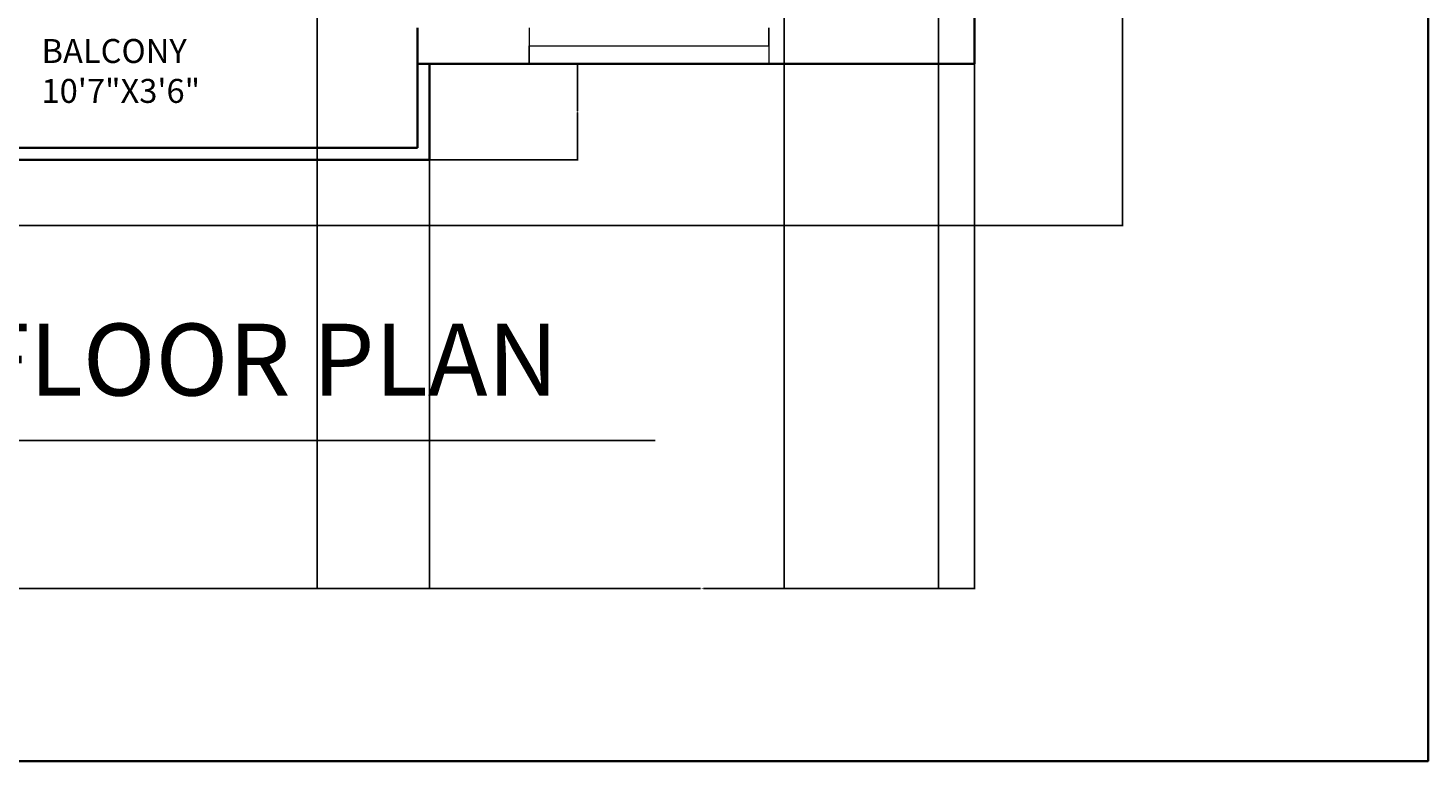
# Model space of a CAD drawing. Units: inches. Extents: x 1854 to 2495, y 1460 to 2772.
# Tile 3 of 12: x 2144 to 2495, y 1460 to 1644. Entities that reach past the tile are written whole.
import ezdxf

# ---------------------------------------------------------------- set-up
doc = ezdxf.new("R2010")
doc.units = ezdxf.units.IN
for name, color, linetype, lineweight in [('A-ANNO-DIMS', 2, 'Continuous', 18), ('A-ANNO-TEXT', 7, 'Continuous', 25), ('A-ANNO-TTLB', 7, 'Continuous', 35), ('A-AREA-IDEN', 7, 'Continuous', 18), ('A-GLAZ', 4, 'Continuous', 18), ('A-WALL', 7, 'Continuous', 35)]:
    doc.layers.add(name, color=color, linetype=linetype, lineweight=lineweight)
doc.styles.get("Standard").update_dxf_attribs({"font": 'arial.ttf'})
doc.dimstyles.get("Standard").update_dxf_attribs({"dimtxt": 0.18, "dimasz": 0.18, "dimexe": 0.18, "dimexo": 0.0625, "dimgap": 0.09, "dimtad": 0, "dimtih": 1, "dimtoh": 1, "dimdec": 4, "dimzin": 0, "dimdsep": 46, "dimtxsty": 'Standard', "dimcen": 0.09, "dimadec": 0, "dimazin": 0, "dimtfac": 1, "dimtdec": 4, "dimtofl": 0, "dimtmove": 0, "dimatfit": 3, "dimfxl": 1, "dimtolj": 1, "dimtzin": 0, "dimarcsym": 0})

# ---------------------------------------------------------------- blocks, each defined once
blk = doc.blocks.new('WINDOW-60IN')
for p, q in [((0, 9), (0, 0)), ((60, 4.5), (60, 9)), ((60, 9), (60, 0)), ((0, 0), (0, 4.5)), ((0, 4.5), (60, 4.5))]:
    blk.add_line(p, q)
blk = doc.blocks.new('*D50')
at = {"layer": 'A-ANNO-DIMS', "color": 0, "lineweight": -2, "transparency": 16777216}
for p, q in [((2381.04, 2272.04), (2418.21, 2272.04)), ((2418.03, 2271.86), (2418.03, 1933.48)), ((2418.03, 1594.72), (2418.03, 1933.11)), ((2119.04, 1594.54), (2418.21, 1594.54))]:
    blk.add_line(p, q, dxfattribs=at)
at = {"layer": 'A-ANNO-DIMS', "color": 0, "transparency": 16777216}
for points in [[(2418, 2271.86), (2418.06, 2271.86), (2418.03, 2272.04)], [(2418, 1594.72), (2418.06, 1594.72), (2418.03, 1594.54)]]:
    blk.add_solid(points, dxfattribs=at)
at = {"layer": 'Defpoints', "color": 0, "transparency": 16777216}
for p in [(2380.98, 2272.04), (2418.03, 2272.04), (2118.98, 1594.54)]:
    blk.add_point(p, dxfattribs=at)
at = {"layer": 'A-ANNO-DIMS', "color": 0, "transparency": 16777216, "insert": (2418.03, 1933.29), "char_height": 0.18, "attachment_point": 5}
blk.add_mtext('\\A1;677.5', dxfattribs=at)
blk = doc.blocks.new('*D59')
at = {"layer": 'A-ANNO-DIMS', "color": 0, "lineweight": -2, "transparency": 16777216}
for p, q in [((2244.48, 1610.98), (2244.48, 1503.44)), ((2118.98, 1594.48), (2118.98, 1503.44)), ((2119.16, 1503.62), (2181.35, 1503.62)), ((2244.3, 1503.62), (2182.12, 1503.62))]:
    blk.add_line(p, q, dxfattribs=at)
at = {"layer": 'A-ANNO-DIMS', "color": 0, "transparency": 16777216}
for points in [[(2119.16, 1503.65), (2119.16, 1503.59), (2118.98, 1503.62)], [(2244.3, 1503.65), (2244.3, 1503.59), (2244.48, 1503.62)]]:
    blk.add_solid(points, dxfattribs=at)
at = {"layer": 'Defpoints', "color": 0, "transparency": 16777216}
for p in [(2244.48, 1611.04), (2118.98, 1594.54), (2244.48, 1503.62)]:
    blk.add_point(p, dxfattribs=at)
at = {"layer": 'A-ANNO-DIMS', "color": 0, "transparency": 16777216, "insert": (2181.73, 1503.62), "char_height": 0.18, "attachment_point": 5}
blk.add_mtext('\\A1;125.5', dxfattribs=at)
blk = doc.blocks.new('*D60')
at = {"layer": 'A-ANNO-DIMS', "color": 0, "lineweight": -2, "transparency": 16777216}
for p, q in [((2380.98, 1634.98), (2380.98, 1503.44)), ((2244.48, 1610.98), (2244.48, 1503.44)), ((2244.66, 1503.62), (2312.35, 1503.62)), ((2380.8, 1503.62), (2313.12, 1503.62))]:
    blk.add_line(p, q, dxfattribs=at)
at = {"layer": 'A-ANNO-DIMS', "color": 0, "transparency": 16777216}
for points in [[(2244.66, 1503.65), (2244.66, 1503.59), (2244.48, 1503.62)], [(2380.8, 1503.65), (2380.8, 1503.59), (2380.98, 1503.62)]]:
    blk.add_solid(points, dxfattribs=at)
at = {"layer": 'Defpoints', "color": 0, "transparency": 16777216}
for p in [(2380.98, 1635.04), (2244.48, 1611.04), (2380.98, 1503.62)]:
    blk.add_point(p, dxfattribs=at)
at = {"layer": 'A-ANNO-DIMS', "color": 0, "transparency": 16777216, "insert": (2312.73, 1503.62), "char_height": 0.18, "attachment_point": 5}
blk.add_mtext('\\A1;136.5', dxfattribs=at)
blk = doc.blocks.new('*D64')
at = {"layer": 'A-ANNO-DIMS', "color": 0, "lineweight": -2, "transparency": 16777216}
for p, q in [((2333.32, 2262.98), (2333.32, 1503.44)), ((2371.98, 2262.98), (2371.98, 1503.44)), ((2333.5, 1503.62), (2352.26, 1503.62)), ((2371.8, 1503.62), (2353.05, 1503.62))]:
    blk.add_line(p, q, dxfattribs=at)
at = {"layer": 'A-ANNO-DIMS', "color": 0, "transparency": 16777216}
for points in [[(2333.5, 1503.65), (2333.5, 1503.59), (2333.32, 1503.62)], [(2371.8, 1503.65), (2371.8, 1503.59), (2371.98, 1503.62)]]:
    blk.add_solid(points, dxfattribs=at)
at = {"layer": 'Defpoints', "color": 0, "transparency": 16777216}
for p in [(2333.32, 2263.04), (2371.98, 2263.04), (2371.98, 1503.62)]:
    blk.add_point(p, dxfattribs=at)
at = {"layer": 'A-ANNO-DIMS', "color": 0, "transparency": 16777216, "insert": (2352.65, 1503.62), "char_height": 0.18, "attachment_point": 5}
blk.add_mtext('\\A1;38.66', dxfattribs=at)
blk = doc.blocks.new('*D70')
at = {"layer": 'A-ANNO-DIMS', "color": 0, "lineweight": -2, "transparency": 16777216}
for p, q in [((2244.54, 1635.04), (2281.71, 1635.04)), ((2281.53, 1634.86), (2281.53, 1623.23)), ((2281.53, 1611.22), (2281.53, 1622.86)), ((2244.54, 1611.04), (2281.71, 1611.04))]:
    blk.add_line(p, q, dxfattribs=at)
at = {"layer": 'A-ANNO-DIMS', "color": 0, "transparency": 16777216}
for points in [[(2281.5, 1634.86), (2281.56, 1634.86), (2281.53, 1635.04)], [(2281.5, 1611.22), (2281.56, 1611.22), (2281.53, 1611.04)]]:
    blk.add_solid(points, dxfattribs=at)
at = {"layer": 'Defpoints', "color": 0, "transparency": 16777216}
for p in [(2244.48, 1635.04), (2244.48, 1611.04), (2281.53, 1611.04)]:
    blk.add_point(p, dxfattribs=at)
at = {"layer": 'A-ANNO-DIMS', "color": 0, "transparency": 16777216, "insert": (2281.53, 1623.04), "char_height": 0.18, "attachment_point": 5}
blk.add_mtext('\\A1;24', dxfattribs=at)
blk = doc.blocks.new('*D73')
at = {"layer": 'A-ANNO-DIMS', "color": 0, "lineweight": -2, "transparency": 16777216}
for p, q in [((2131.08, 2220.98), (2131.08, 1503.44)), ((2216.32, 2220.98), (2216.32, 1503.44)), ((2131.26, 1503.62), (2173.31, 1503.62)), ((2216.14, 1503.62), (2174.1, 1503.62))]:
    blk.add_line(p, q, dxfattribs=at)
at = {"layer": 'A-ANNO-DIMS', "color": 0, "transparency": 16777216}
for points in [[(2131.26, 1503.65), (2131.26, 1503.59), (2131.08, 1503.62)], [(2216.14, 1503.65), (2216.14, 1503.59), (2216.32, 1503.62)]]:
    blk.add_solid(points, dxfattribs=at)
at = {"layer": 'Defpoints', "color": 0, "transparency": 16777216}
for p in [(2131.08, 2221.04), (2216.32, 2221.04), (2216.32, 1503.62)]:
    blk.add_point(p, dxfattribs=at)
at = {"layer": 'A-ANNO-DIMS', "color": 0, "transparency": 16777216, "insert": (2173.7, 1503.62), "char_height": 0.18, "attachment_point": 5}
blk.add_mtext('\\A1;85.25', dxfattribs=at)

msp = doc.modelspace()

# ---------------------------------------------------------------- linework, layer by layer
at = {"layer": 'A-ANNO-TEXT'}
msp.add_line((2054.5799, 1540.6707), (2301.0328, 1540.6707), dxfattribs=at)
at = {"layer": 'A-ANNO-TTLB'}
msp.add_lwpolyline([(1854.1764, 2772.4852), (2494.521, 2772.4852), (2494.521, 1460.4076), (1854.1764, 1460.4076)], close=True, dxfattribs=at)
at = {"layer": 'A-WALL'}
for p, q in [((2380.9824, 1635.0449), (2380.9824, 1652.2587)), ((2241.4824, 1644.0449), (2241.4824, 1635.0449)), ((2241.4824, 1635.0449), (2380.9824, 1635.0449)), ((2241.4824, 1635.0449), (2241.4824, 1617.0449)), ((2241.4824, 1635.0449), (2244.4824, 1635.0449)), ((2244.4824, 1635.0449), (2244.4824, 1614.0449)), ((2241.4824, 1617.0449), (2241.4824, 1614.0449)), ((2241.4824, 1614.0449), (2118.9824, 1614.0449)), ((2244.4824, 1614.0449), (2244.4824, 1611.0449)), ((2244.4824, 1611.0449), (2118.9824, 1611.0449))]:
    msp.add_line(p, q, dxfattribs=at)

# ---------------------------------------------------------------- block references
at = {"layer": 'A-GLAZ'}
msp.add_blockref('WINDOW-60IN', (2269.4453, 1635.045), dxfattribs=at)

# ---------------------------------------------------------------- texts
at = {"layer": 'A-ANNO-TEXT', "insert": (2059.5829, 1569.9747), "char_height": 18, "attachment_point": 1}
msp.add_mtext_dynamic_manual_height_columns('FIRST FLOOR PLAN', width=268.218755, gutter_width=12.5, heights=[0], dxfattribs=at)
at = {"layer": 'A-AREA-IDEN', "insert": (2147.3322, 1641.283), "char_height": 6, "attachment_point": 1}
msp.add_mtext_dynamic_manual_height_columns('BALCONY\\P10\'7"X3\'6"', width=112.404111, gutter_width=12.5, heights=[0], dxfattribs=at)

# ---------------------------------------------------------------- dimensions: what is measured, and where the dimension line sits
at = {"layer": 'A-ANNO-DIMS'}
for base, p1, p2, angle, override, picture, middle in [((2418.0324, 2272.0449), (2118.9824, 1594.5449), (2380.9824, 2272.0449), 90, {"dimdec": 1, "dimlfac": 1, "dimrnd": 0, "dimzin": 0, "dimdsep": 46, "dimlunit": 2}, '*D50', (2418.0324, 1933.2949)), ((2281.5324, 1611.0449), (2244.4824, 1635.0449), (2244.4824, 1611.0449), 270, {"dimdec": 0, "dimlfac": 1, "dimrnd": 0, "dimzin": 0, "dimdsep": 46, "dimlunit": 2}, '*D70', (2281.5324, 1623.0449))]:
    dim = msp.add_linear_dim(base=base, p1=p1, p2=p2, angle=angle, dimstyle='Standard', override=override, dxfattribs=at)
    dim.commit()
    dim.dimension.update_dxf_attribs({"geometry": picture, "text_midpoint": middle})
for base, p1, p2, override, picture, middle in [((2371.9824, 1503.6207), (2333.3214, 2263.0449), (2371.9824, 2263.0449), {"dimdec": 2, "dimlfac": 1, "dimrnd": 0, "dimzin": 0, "dimdsep": 46, "dimlunit": 2}, '*D64', (2352.6519, 1503.6207)), ((2216.3239, 1503.6207), (2131.0775, 2221.0449), (2216.3239, 2221.0449), {"dimdec": 2, "dimlfac": 1, "dimrnd": 0, "dimzin": 0, "dimdsep": 46, "dimlunit": 2}, '*D73', (2173.7007, 1503.6207)), ((2380.9824, 1503.6207), (2244.4824, 1611.0449), (2380.9824, 1635.0449), {"dimdec": 1, "dimlfac": 1, "dimrnd": 0, "dimzin": 0, "dimdsep": 46, "dimlunit": 2}, '*D60', (2312.7324, 1503.6207)), ((2244.4824, 1503.6207), (2118.9824, 1594.5449), (2244.4824, 1611.0449), {"dimdec": 1, "dimlfac": 1, "dimrnd": 0, "dimzin": 0, "dimdsep": 46, "dimlunit": 2}, '*D59', (2181.7324, 1503.6207))]:
    dim = msp.add_linear_dim(base=base, p1=p1, p2=p2, dimstyle='Standard', override=override, dxfattribs=at)
    dim.commit()
    dim.dimension.update_dxf_attribs({"geometry": picture, "text_midpoint": middle})

doc.saveas('drawing.dxf')
